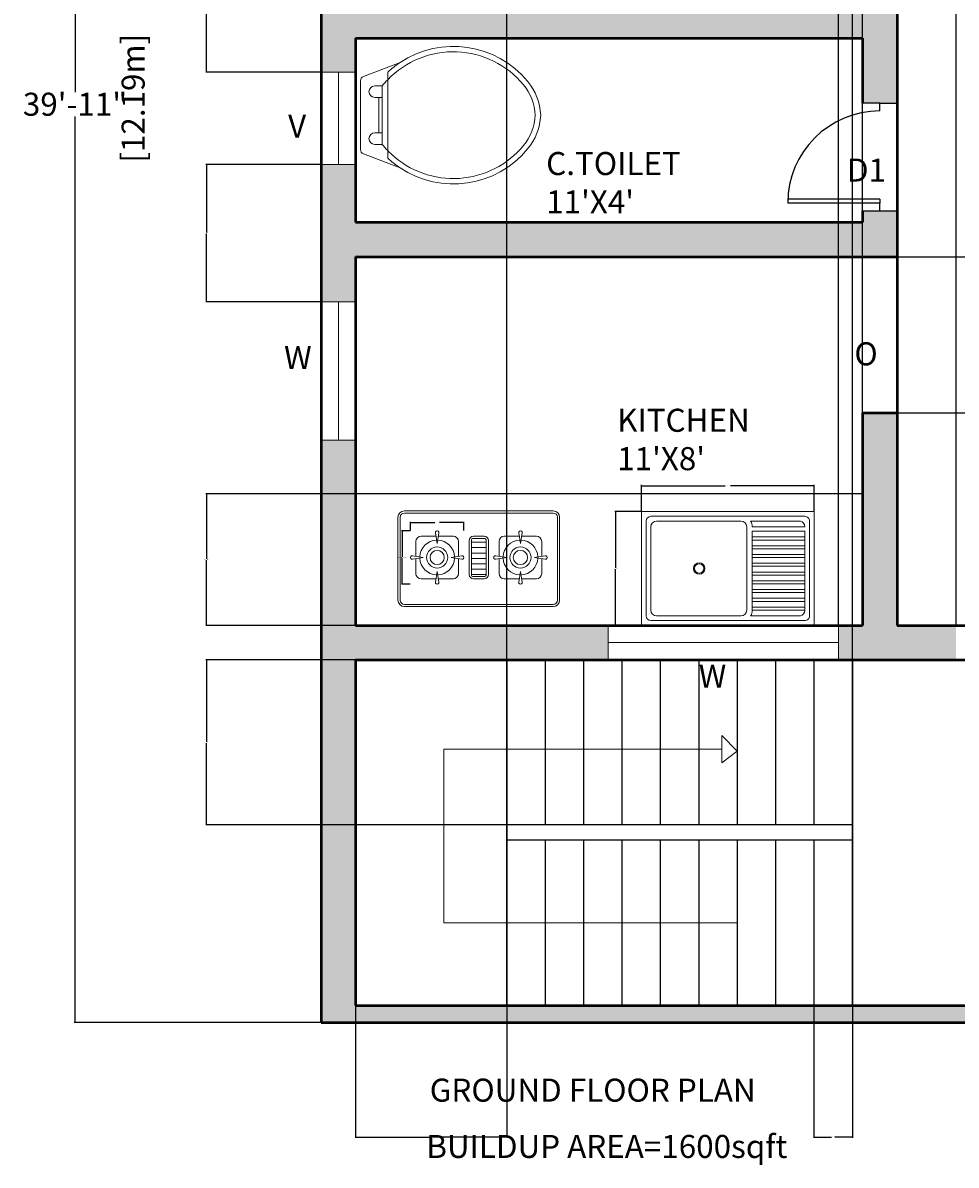
# Model space of a CAD drawing. Units: inches. Extents: x -55 to 413, y -498 to 86.
# Tile 1 of 6: x -55 to 188, y -498 to -201. Entities that reach past the tile are written whole.
import ezdxf

# ---------------------------------------------------------------- set-up
doc = ezdxf.new("R2010")
doc.units = ezdxf.units.IN
doc.header["$MEASUREMENT"] = 0
for name, color, linetype, lineweight in [('A-ANNO-DIMS', 2, 'Continuous', 18), ('A-ANNO-SYMB', 7, 'Continuous', 18), ('A-ANNO-TEXT', 7, 'Continuous', 25), ('A-AREA-IDEN', 7, 'Continuous', 25), ('A-DOOR', 3, 'Continuous', 25), ('A-EQPM', 9, 'Continuous', 18), ('A-EQPM-PATT', 9, 'Continuous', 13), ('A-FLOR-CASE', 7, 'Continuous', 25), ('A-FLOR-FIXT', 9, 'Continuous', 18), ('A-FLOR-STRS', 7, 'Continuous', 25), ('A-GLAZ', 4, 'Continuous', 18), ('A-WALL', 7, 'Continuous', 50), ('A-WALL-PATT', 8, 'Continuous', 13)]:
    doc.layers.add(name, color=color, linetype=linetype, lineweight=lineweight)
doc.styles.get("Standard").update_dxf_attribs({"font": 'arial.ttf'})
doc.dimstyles.get("Standard").update_dxf_attribs({"dimtxt": 0.18, "dimasz": 0.18, "dimexe": 0.18, "dimexo": 0.0625, "dimgap": 0.09, "dimtad": 0, "dimtih": 1, "dimtoh": 1, "dimdec": 0, "dimzin": 0, "dimdsep": 46, "dimlunit": 3, "dimtxsty": 'Standard', "dimcen": 0.09, "dimadec": 0, "dimazin": 0, "dimtfac": 1, "dimtdec": 0, "dimtofl": 0, "dimtmove": 0, "dimatfit": 3, "dimfxl": 1, "dimtolj": 1, "dimtzin": 0, "dimarcsym": 0})

# ---------------------------------------------------------------- blocks, each defined once
blk = doc.blocks.new('М12 540х820')
for p, q in [((0, 540), (-820, 540)), ((-820, 540), (-820, 0)), ((-797.5, 495), (-797.5, 45)), ((-45, 517.5), (-775, 517.5)), ((-347.5, 495), (-748, 495)), ((-301.7, 495), (-64.8, 495)), ((-22.5, 45), (-22.5, 495)), ((0, 0), (0, 540)), ((-775, 468), (-775, 72)), ((-320.5, 468), (-320.5, 72)), ((-293.7, 468), (-293.7, 472.5)), ((-293.7, 468), (-45, 468)), ((-293.7, 446.6), (-45, 446.6)), ((-293.7, 419.6), (-293.7, 446.6)), ((-45, 469.5), (-45, 468)), ((-45, 419.6), (-45, 446.6)), ((-293.7, 419.6), (-45, 419.6)), ((-293.7, 405), (-45, 405)), ((-293.7, 378), (-293.7, 405)), ((-45, 378), (-45, 405)), ((-293.7, 378), (-45, 378)), ((-293.7, 336.4), (-293.7, 363.4)), ((-293.7, 363.4), (-45, 363.4)), ((-293.7, 336.4), (-45, 336.4)), ((-45, 336.4), (-45, 363.4)), ((-293.7, 294.7), (-293.7, 321.7)), ((-293.7, 321.7), (-45, 321.7)), ((-293.7, 294.7), (-45, 294.7)), ((-293.7, 253.1), (-293.7, 280.1)), ((-293.7, 280.1), (-45, 280.1)), ((-45, 294.7), (-45, 321.7)), ((-45, 253.1), (-45, 280.1)), ((-293.7, 253.1), (-45, 253.1)), ((-293.7, 211.5), (-293.7, 238.5)), ((-293.7, 238.5), (-45, 238.5)), ((-45, 211.5), (-45, 238.5)), ((-293.7, 211.5), (-45, 211.5)), ((-293.7, 169.9), (-293.7, 196.9)), ((-293.7, 196.9), (-45, 196.9)), ((-293.7, 169.9), (-45, 169.9)), ((-45, 169.9), (-45, 196.9)), ((-293.7, 128.2), (-293.7, 155.2)), ((-293.7, 155.2), (-45, 155.2)), ((-293.7, 128.2), (-45, 128.2)), ((-293.7, 113.6), (-45, 113.6)), ((-293.7, 86.6), (-293.7, 113.6)), ((-45, 128.2), (-45, 155.2)), ((-45, 86.6), (-45, 113.6)), ((-293.7, 86.6), (-45, 86.6)), ((-293.7, 72), (-45, 72)), ((-45, 70.5), (-45, 72)), ((-820, 0), (0, 0)), ((-775, 22.5), (-45, 22.5)), ((-748, 45), (-347.5, 45)), ((-301.7, 45), (-64.8, 45))]:
    blk.add_line(p, q)
at = {"ltscale": 0.06}
for p, q in [((-820, 0), (-820, 540)), ((-820, 540), (0, 540)), ((0, 540), (0, 536.9)), ((0, 536.9), (0, 0)), ((-293.7, 446.6), (-45, 446.6)), ((-293.7, 405), (-293.7, 446.6)), ((-45, 446.6), (-45, 419.6)), ((-293.7, 363.4), (-293.7, 405)), ((-45, 419.6), (-45, 378)), ((-293.7, 321.7), (-293.7, 363.4)), ((-45, 378), (-45, 336.4)), ((-45, 336.4), (-45, 294.7)), ((-293.7, 280.1), (-293.7, 321.7)), ((-293.7, 238.5), (-293.7, 280.1)), ((-45, 294.7), (-45, 253.1)), ((-293.7, 196.9), (-293.7, 238.5)), ((-45, 253.1), (-45, 211.5)), ((-293.7, 155.2), (-293.7, 196.9)), ((-45, 211.5), (-45, 169.9)), ((-45, 169.9), (-45, 128.2)), ((-293.7, 113.6), (-293.7, 155.2)), ((-293.7, 72), (-293.7, 113.6)), ((-45, 128.2), (-45, 86.6)), ((-45, 72), (-293.7, 72)), ((-45, 86.6), (-45, 72)), ((0, 0), (-820, 0))]:
    blk.add_line(p, q, dxfattribs=at)
at = {"extrusion": (0, 0, -1)}
for centre, major_axis, start_param, end_param in [((-775, 495), (-15.9, 15.9), -0.785398, 0.785398), ((-775, 495), (-15.9, 15.9), -0.785398, 0.785398), ((-748, 468), (-19.1, -19.1), 0.785398, 2.356194), ((-748, 468), (-19.1, -19.1), 0.785398, 2.356194), ((-347.5, 468), (-19.1, 19.1), 0.785398, 2.356194), ((-347.5, 468), (-19.1, 19.1), 0.785398, 2.356194), ((-343.2, 468), (-35, 35), 1.779263, 2.356194), ((-343.2, 468), (-35, 35), 1.779263, 2.356192), ((-72.3, 468.8), (-19.3, 19.3), 1.0328, 2.38382), ((-72.3, 468.8), (-19.3, 19.3), 1.0328, 1.064673), ((-72.3, 468.8), (-19.3, 19.3), 1.064673, 2.328569), ((-45, 495), (-15.9, -15.9), 2.356194, 3.926991), ((-45, 495), (-15.9, -15.9), 2.356194, 3.926991), ((-343.2, 468), (-35, 35), 2.356192, 2.356194), ((-72.3, 468.8), (-19.3, 19.3), 2.328569, 2.38382), ((-545.5, 270), (-19.1, -19.1), 3.926991, 10.210176), ((-545.5, 270), (-19.1, -19.1), 3.926991, 10.210176), ((-545.5, 270), (-15.9, -15.9), 3.926991, 10.210176), ((-545.5, 270), (-15.9, -15.9), 3.926991, 10.210176), ((-748, 72), (-19.1, 19.1), 3.926991, 5.497787), ((-748, 72), (-19.1, 19.1), 3.926991, 5.497787), ((-347.5, 72), (-19.1, -19.1), 3.926991, 5.497787), ((-347.5, 72), (-19.1, -19.1), 3.926991, 5.497787), ((-343.2, 72), (-35, -35), 3.926991, 4.503922), ((-343.2, 72), (-35, -35), 3.926991, 4.503922), ((-72.3, 71.2), (-19.3, -19.3), 3.899365, 5.250385), ((-72.3, 71.2), (-19.3, -19.3), 3.954617, 5.218512), ((-72.3, 71.2), (-19.3, -19.3), 3.899365, 3.954617), ((-775, 45), (-15.9, -15.9), 5.497787, 7.068583), ((-775, 45), (-15.9, -15.9), 5.497787, 7.068583), ((-72.3, 71.2), (-19.3, -19.3), 5.218512, 5.250385), ((-45, 45), (-15.9, 15.9), 2.356194, 3.926991), ((-45, 45), (-15.9, 15.9), 2.356194, 3.926991)]:
    blk.add_ellipse(centre, major_axis=major_axis, ratio=1, start_param=start_param, end_param=end_param, dxfattribs=at)
blk = doc.blocks.new('*D3')
at = {"layer": 'A-ANNO-DIMS', "color": 0, "lineweight": -2, "transparency": 16777216}
for p, q in [((22.94, 17.54), (-41.24, 17.54)), ((-41.06, 17.36), (-41.06, -218.55)), ((-41.06, -460.78), (-41.06, -224.87)), ((22.94, -460.96), (-41.24, -460.96))]:
    blk.add_line(p, q, dxfattribs=at)
at = {"layer": 'A-ANNO-DIMS', "color": 0, "transparency": 16777216}
for points in [[(-41.09, 17.36), (-41.03, 17.36), (-41.06, 17.54)], [(-41.09, -460.78), (-41.03, -460.78), (-41.06, -460.96)]]:
    blk.add_solid(points, dxfattribs=at)
at = {"layer": 'Defpoints', "color": 0, "transparency": 16777216}
for p in [(23, 17.54), (-41.06, -460.96), (23, -460.96)]:
    blk.add_point(p, dxfattribs=at)
at = {"layer": 'A-ANNO-DIMS', "color": 0, "transparency": 16777216, "insert": (-41.06, -221.71), "char_height": 6, "attachment_point": 5}
blk.add_mtext('\\A1;39\'-11"', dxfattribs=at)
blk = doc.blocks.new('WC-PLAN')
for p, q in [((7.1, 27.15), (7.1, 29.12)), ((7.1, 27.15), (7.1, 17.92)), ((7.1, 8.69), (7.1, 17.92)), ((7.1, 6.73), (7.1, 8.69))]:
    blk.add_line(p, q)
for points in [[(10.32, 31.66, -0.383919), (43.53, 26.74, -0.163732), (46.92, 17.92, -0.359733)], [(7.1, 27.15, -0.448546), (42.45, 25.85, -0.162618), (45.51, 17.92, -0.470877)], [(0, 17.92), (0, 26.88, -0.31031), (0.75, 27.98), (10.32, 31.66, -0.209071)], [(7.1, 29.12, -0.040937), (10.32, 31.66, -0.163732)], [(5.69, 25.54, -0.022712), (7.1, 27.15, -0.162618)], [(5.69, 25.54), (3.72, 25.54, 1), (3.72, 22.54), (4.74, 22.54)], [(5.69, 17.92), (5.69, 25.54, -0.476108)], [(0, 17.92), (0, 8.97, 0.31031), (0.75, 7.87), (10.32, 4.19, 0.209071)], [(5.69, 17.92), (5.69, 10.31, 0.022712)], [(8.06, 7.75, 0.431639), (42.45, 10, 0.162618), (45.51, 17.92, 0.470877)], [(10.32, 4.19, 0.383919), (43.53, 9.11, 0.163732), (46.92, 17.92, 0.359733)], [(5.69, 10.31), (3.72, 10.31, -1), (3.72, 13.31), (4.74, 13.31)], [(5.69, 10.31, 0.022712), (7.1, 8.69, 0.162618)], [(7.1, 8.69, 0.014165), (8.06, 7.75, 0.162618)], [(7.1, 6.73, 0.040937), (10.32, 4.19, 0.163732)]]:
    blk.add_lwpolyline(points, format="xyb")
for points in [[(4.74, 22.54), (4.74, 13.31)], [(4.74, 22.54), (5.69, 22.54)], [(4.74, 13.31), (5.69, 13.31)]]:
    blk.add_lwpolyline(points)
blk = doc.blocks.new('DOOR-SINGLE-24')
for p, q in [((24, 28), (19.5, 28)), ((24, 26), (24, 28)), ((24, 28), (28.5, 28)), ((24, 3), (0, 3)), ((24, 3), (24, 2)), ((24, 2), (0, 2)), ((24, 0), (24, 2)), ((19.5, 0), (28.5, 0))]:
    blk.add_line(p, q)
blk.add_arc((24, 2), 24, 90, 180)
blk = doc.blocks.new('COOKTOP-BURNER')
for p, q in [((6.66, 12.49), (2.75, 12.49)), ((6.52, 13.4), (6.96, 10.59)), ((6.96, 10.59), (7.4, 13.4)), ((11.17, 12.49), (7.26, 12.49)), ((1.42, 11.17), (1.42, 7.26)), ((12.5, 7.26), (12.5, 11.17)), ((0.52, 7.4), (3.33, 6.96)), ((3.33, 6.96), (0.52, 6.52)), ((1.42, 6.66), (1.42, 2.75)), ((13.4, 7.4), (10.59, 6.96)), ((10.59, 6.96), (13.4, 6.52)), ((12.5, 2.75), (12.5, 6.66)), ((6.52, 0.52), (6.96, 3.33)), ((6.96, 3.33), (7.4, 0.52)), ((2.75, 1.42), (6.66, 1.42)), ((7.26, 1.42), (11.17, 1.42))]:
    blk.add_line(p, q)
for radius in [2.75, 1.86]:
    blk.add_circle((6.96, 6.96), radius)
for centre, radius, start, end in [((2.75, 11.17), 1.33, 90, 180), ((6.96, 13.47), 0.448, 351.0363, 188.9637), ((11.17, 11.17), 1.33, 0, 90), ((6.96, 6.96), 4.52, 91.7678, 178.2322), ((6.96, 6.96), 4.52, 1.7678, 88.2322), ((0.45, 6.96), 0.448, 81.0363, 278.9637), ((6.96, 6.96), 4.52, 181.7678, 268.2322), ((6.96, 6.96), 4.52, 271.7678, 358.2322), ((13.47, 6.96), 0.448, 261.0363, 98.9637), ((2.75, 2.75), 1.33, 180, 270), ((6.96, 0.45), 0.448, 171.0363, 8.9637), ((11.17, 2.75), 1.33, 270, 0)]:
    blk.add_arc(centre, radius, start, end)
blk = doc.blocks.new('WIN-60IN')
for p, q in [((0, 9), (60, 9)), ((0, 0), (0, 9)), ((60, 9), (60, 0)), ((0, 4.5), (60, 4.5)), ((60, 0), (0, 0))]:
    blk.add_line(p, q)
blk = doc.blocks.new('WIN-24IN')
for p, q in [((24, 9), (0, 9)), ((0, 9), (0, 0)), ((24, 0), (24, 9)), ((0, 4.5), (24, 4.5)), ((0, 0), (24, 0))]:
    blk.add_line(p, q)
blk = doc.blocks.new('WIN-36IN')
for p, q in [((0, 36), (0, 0)), ((9, 36), (0, 36)), ((4.5, 36), (4.5, 0)), ((9, 0), (9, 36)), ((0, 0), (9, 0))]:
    blk.add_line(p, q)
blk = doc.blocks.new('*D23')
at = {"layer": 'A-ANNO-DIMS', "color": 0, "lineweight": -2, "transparency": 16777216}
for p, q in [((46.18, -332.81), (43.97, -332.81)), ((44.15, -332.99), (44.15, -339.61)), ((44.15, -346.59), (44.15, -339.97)), ((46.18, -346.77), (43.97, -346.77))]:
    blk.add_line(p, q, dxfattribs=at)
at = {"layer": 'A-ANNO-DIMS', "color": 0, "transparency": 16777216}
for points in [[(44.12, -332.99), (44.18, -332.99), (44.15, -332.81)], [(44.12, -346.59), (44.18, -346.59), (44.15, -346.77)]]:
    blk.add_solid(points, dxfattribs=at)
at = {"layer": 'Defpoints', "color": 0, "transparency": 16777216}
for p in [(44.15, -332.81), (46.25, -332.81), (46.25, -346.77)]:
    blk.add_point(p, dxfattribs=at)
at = {"layer": 'A-ANNO-DIMS', "color": 0, "transparency": 16777216, "insert": (44.15, -339.79), "char_height": 0.18, "attachment_point": 5}
blk.add_mtext('\\A1;BURNER 1\'-2" TYP.', dxfattribs=at)
blk = doc.blocks.new('*D24')
at = {"layer": 'A-ANNO-DIMS', "color": 0, "lineweight": -2, "transparency": 16777216}
for p, q in [((46.25, -332.75), (46.25, -330.53)), ((46.43, -330.71), (52.6, -330.71)), ((60.03, -330.71), (53.86, -330.71)), ((60.21, -332.75), (60.21, -330.53))]:
    blk.add_line(p, q, dxfattribs=at)
at = {"layer": 'A-ANNO-DIMS', "color": 0, "transparency": 16777216}
for points in [[(46.43, -330.68), (46.43, -330.74), (46.25, -330.71)], [(60.03, -330.68), (60.03, -330.74), (60.21, -330.71)]]:
    blk.add_solid(points, dxfattribs=at)
at = {"layer": 'Defpoints', "color": 0, "transparency": 16777216}
for p in [(46.25, -332.81), (60.21, -330.71), (60.21, -332.81)]:
    blk.add_point(p, dxfattribs=at)
at = {"layer": 'A-ANNO-DIMS', "color": 0, "transparency": 16777216, "insert": (53.23, -330.71), "char_height": 0.18, "attachment_point": 5}
blk.add_mtext('\\A1;1\'-2" TYP.', dxfattribs=at)
blk = doc.blocks.new('*D25')
at = {"layer": 'A-ANNO-DIMS', "color": 0, "lineweight": -2, "transparency": 16777216}
for p, q in [((106.4, -327.76), (106.4, -320.9)), ((106.58, -321.08), (128.24, -321.08)), ((151.22, -321.08), (129.56, -321.08)), ((151.4, -327.76), (151.4, -320.9))]:
    blk.add_line(p, q, dxfattribs=at)
at = {"layer": 'A-ANNO-DIMS', "color": 0, "transparency": 16777216}
for points in [[(106.58, -321.05), (106.58, -321.11), (106.4, -321.08)], [(151.22, -321.05), (151.22, -321.11), (151.4, -321.08)]]:
    blk.add_solid(points, dxfattribs=at)
at = {"layer": 'Defpoints', "color": 0, "transparency": 16777216}
for p in [(151.4, -321.08), (106.4, -327.83), (151.4, -327.83)]:
    blk.add_point(p, dxfattribs=at)
at = {"layer": 'A-ANNO-DIMS', "color": 0, "transparency": 16777216, "insert": (128.9, -321.08), "char_height": 0.18, "attachment_point": 5}
blk.add_mtext('\\A1;SINK 3\'-9"', dxfattribs=at)
blk = doc.blocks.new('*D26')
at = {"layer": 'A-ANNO-DIMS', "color": 0, "lineweight": -2, "transparency": 16777216}
for p, q in [((106.34, -327.83), (99.47, -327.83)), ((99.65, -328.01), (99.65, -342.46)), ((99.65, -357.28), (99.65, -342.83)), ((106.34, -357.46), (99.47, -357.46))]:
    blk.add_line(p, q, dxfattribs=at)
at = {"layer": 'A-ANNO-DIMS', "color": 0, "transparency": 16777216}
for points in [[(99.62, -328.01), (99.68, -328.01), (99.65, -327.83)], [(99.62, -357.28), (99.68, -357.28), (99.65, -357.46)]]:
    blk.add_solid(points, dxfattribs=at)
at = {"layer": 'Defpoints', "color": 0, "transparency": 16777216}
for p in [(99.65, -327.83), (106.4, -327.83), (106.4, -357.46)]:
    blk.add_point(p, dxfattribs=at)
at = {"layer": 'A-ANNO-DIMS', "color": 0, "transparency": 16777216, "insert": (99.65, -342.64), "char_height": 0.18, "attachment_point": 5}
blk.add_mtext('\\A1;2\'-5 1/2"', dxfattribs=at)
blk = doc.blocks.new('*D31')
at = {"layer": 'A-ANNO-DIMS', "color": 0, "lineweight": -2, "transparency": 16777216}
for p, q in [((22.94, -237.4), (-6.98, -237.4)), ((-6.8, -237.58), (-6.8, -255.13)), ((-6.8, -273.04), (-6.8, -255.5)), ((22.94, -273.22), (-6.98, -273.22))]:
    blk.add_line(p, q, dxfattribs=at)
at = {"layer": 'A-ANNO-DIMS', "color": 0, "transparency": 16777216}
for points in [[(-6.83, -237.58), (-6.77, -237.58), (-6.8, -237.4)], [(-6.83, -273.04), (-6.77, -273.04), (-6.8, -273.22)]]:
    blk.add_solid(points, dxfattribs=at)
at = {"layer": 'Defpoints', "color": 0, "transparency": 16777216}
for p in [(23, -237.4), (-6.8, -273.22), (23, -273.22)]:
    blk.add_point(p, dxfattribs=at)
at = {"layer": 'A-ANNO-DIMS', "color": 0, "transparency": 16777216, "insert": (-6.8, -255.31), "char_height": 0.18, "attachment_point": 5}
blk.add_mtext('\\A1;3\'-0"', dxfattribs=at)
blk = doc.blocks.new('*D32')
at = {"layer": 'A-ANNO-DIMS', "color": 0, "lineweight": -2, "transparency": 16777216}
for p, q in [((22.94, -154.08), (-6.98, -154.08)), ((-6.8, -154.26), (-6.8, -183.56)), ((-6.8, -213.22), (-6.8, -183.93)), ((22.94, -213.4), (-6.98, -213.4))]:
    blk.add_line(p, q, dxfattribs=at)
at = {"layer": 'A-ANNO-DIMS', "color": 0, "transparency": 16777216}
for points in [[(-6.83, -154.26), (-6.77, -154.26), (-6.8, -154.08)], [(-6.83, -213.22), (-6.77, -213.22), (-6.8, -213.4)]]:
    blk.add_solid(points, dxfattribs=at)
at = {"layer": 'Defpoints', "color": 0, "transparency": 16777216}
for p in [(23, -154.08), (-6.8, -213.4), (23, -213.4)]:
    blk.add_point(p, dxfattribs=at)
at = {"layer": 'A-ANNO-DIMS', "color": 0, "transparency": 16777216, "insert": (-6.8, -183.74), "char_height": 0.18, "attachment_point": 5}
blk.add_mtext('\\A1;4\'-11 1/2"', dxfattribs=at)
blk = doc.blocks.new('*D35')
at = {"layer": 'A-ANNO-DIMS', "color": 0, "lineweight": -2, "transparency": 16777216}
for p, q in [((164.07, -261.46), (412.98, -261.46)), ((412.8, -261.64), (412.8, -281.58)), ((412.8, -301.89), (412.8, -281.95)), ((164.07, -302.07), (412.98, -302.07))]:
    blk.add_line(p, q, dxfattribs=at)
at = {"layer": 'A-ANNO-DIMS', "color": 0, "transparency": 16777216}
for points in [[(412.77, -261.64), (412.83, -261.64), (412.8, -261.46)], [(412.77, -301.89), (412.83, -301.89), (412.8, -302.07)]]:
    blk.add_solid(points, dxfattribs=at)
at = {"layer": 'Defpoints', "color": 0, "transparency": 16777216}
for p in [(164, -261.46), (412.8, -261.46), (164, -302.07)]:
    blk.add_point(p, dxfattribs=at)
at = {"layer": 'A-ANNO-DIMS', "color": 0, "transparency": 16777216, "insert": (412.8, -281.76), "char_height": 0.18, "attachment_point": 5}
blk.add_mtext('\\A1;3\'-4 1/2"', dxfattribs=at)
blk = doc.blocks.new('*D40')
at = {"layer": 'A-ANNO-DIMS', "color": 0, "lineweight": -2, "transparency": 16777216}
for p, q in [((157.71, -357.4), (157.71, 47.52)), ((157.89, 47.34), (160.32, 47.34)), ((163.82, 47.34), (161.39, 47.34)), ((164, -357.4), (164, 47.52))]:
    blk.add_line(p, q, dxfattribs=at)
at = {"layer": 'A-ANNO-DIMS', "color": 0, "transparency": 16777216}
for points in [[(157.89, 47.37), (157.89, 47.31), (157.71, 47.34)], [(163.82, 47.37), (163.82, 47.31), (164, 47.34)]]:
    blk.add_solid(points, dxfattribs=at)
at = {"layer": 'Defpoints', "color": 0, "transparency": 16777216}
for p in [(164, 47.34), (157.71, -357.46), (164, -357.46)]:
    blk.add_point(p, dxfattribs=at)
at = {"layer": 'A-ANNO-DIMS', "color": 0, "transparency": 16777216, "insert": (160.86, 47.34), "char_height": 0.18, "attachment_point": 5}
blk.add_mtext('\\A1;0\'-6 1/2"', dxfattribs=at)
blk = doc.blocks.new('*D41')
at = {"layer": 'A-ANNO-DIMS', "color": 0, "lineweight": -2, "transparency": 16777216}
for p, q in [((173, -357.4), (173, 47.52)), ((173.18, 47.34), (180.15, 47.34)), ((188.17, 47.34), (181.21, 47.34)), ((188.35, -357.4), (188.35, 47.52))]:
    blk.add_line(p, q, dxfattribs=at)
at = {"layer": 'A-ANNO-DIMS', "color": 0, "transparency": 16777216}
for points in [[(173.18, 47.37), (173.18, 47.31), (173, 47.34)], [(188.17, 47.37), (188.17, 47.31), (188.35, 47.34)]]:
    blk.add_solid(points, dxfattribs=at)
at = {"layer": 'Defpoints', "color": 0, "transparency": 16777216}
for p in [(188.35, 47.34), (173, -357.46), (188.35, -357.46)]:
    blk.add_point(p, dxfattribs=at)
at = {"layer": 'A-ANNO-DIMS', "color": 0, "transparency": 16777216, "insert": (180.68, 47.34), "char_height": 0.18, "attachment_point": 5}
blk.add_mtext('\\A1;1\'-3 1/2"', dxfattribs=at)
blk = doc.blocks.new('*D43')
at = {"layer": 'A-ANNO-DIMS', "color": 0, "lineweight": -2, "transparency": 16777216}
for p, q in [((71.33, -456.4), (71.33, 47.52)), ((71.51, 47.34), (116, 47.34)), ((161.15, 47.34), (116.66, 47.34)), ((161.33, -456.4), (161.33, 47.52))]:
    blk.add_line(p, q, dxfattribs=at)
at = {"layer": 'A-ANNO-DIMS', "color": 0, "transparency": 16777216}
for points in [[(71.51, 47.37), (71.51, 47.31), (71.33, 47.34)], [(161.15, 47.37), (161.15, 47.31), (161.33, 47.34)]]:
    blk.add_solid(points, dxfattribs=at)
at = {"layer": 'Defpoints', "color": 0, "transparency": 16777216}
for p in [(161.33, 47.34), (71.33, -456.46), (161.33, -456.46)]:
    blk.add_point(p, dxfattribs=at)
at = {"layer": 'A-ANNO-DIMS', "color": 0, "transparency": 16777216, "insert": (116.33, 47.34), "char_height": 0.18, "attachment_point": 5}
blk.add_mtext('\\A1;7\'-6"', dxfattribs=at)
blk = doc.blocks.new('*D44')
at = {"layer": 'A-ANNO-DIMS', "color": 0, "lineweight": -2, "transparency": 16777216}
for p, q in [((32, -456.52), (32, -490.94)), ((71.33, -456.52), (71.33, -490.94)), ((32.18, -490.76), (51.13, -490.76)), ((71.15, -490.76), (52.21, -490.76))]:
    blk.add_line(p, q, dxfattribs=at)
at = {"layer": 'A-ANNO-DIMS', "color": 0, "transparency": 16777216}
for points in [[(32.18, -490.73), (32.18, -490.79), (32, -490.76)], [(71.15, -490.73), (71.15, -490.79), (71.33, -490.76)]]:
    blk.add_solid(points, dxfattribs=at)
at = {"layer": 'Defpoints', "color": 0, "transparency": 16777216}
for p in [(32, -456.46), (71.33, -456.46), (71.33, -490.76)]:
    blk.add_point(p, dxfattribs=at)
at = {"layer": 'A-ANNO-DIMS', "color": 0, "transparency": 16777216, "insert": (51.67, -490.76), "char_height": 0.18, "attachment_point": 5}
blk.add_mtext('\\A1;3\'-3 1/2"', dxfattribs=at)
blk = doc.blocks.new('*D45')
at = {"layer": 'A-ANNO-DIMS', "color": 0, "lineweight": -2, "transparency": 16777216}
for p, q in [((151.33, -456.52), (151.33, -490.94)), ((161.33, -456.52), (161.33, -490.94)), ((151.51, -490.76), (155.93, -490.76)), ((161.15, -490.76), (156.73, -490.76))]:
    blk.add_line(p, q, dxfattribs=at)
at = {"layer": 'A-ANNO-DIMS', "color": 0, "transparency": 16777216}
for points in [[(151.51, -490.73), (151.51, -490.79), (151.33, -490.76)], [(161.15, -490.73), (161.15, -490.79), (161.33, -490.76)]]:
    blk.add_solid(points, dxfattribs=at)
at = {"layer": 'Defpoints', "color": 0, "transparency": 16777216}
for p in [(151.33, -456.46), (161.33, -456.46), (161.33, -490.76)]:
    blk.add_point(p, dxfattribs=at)
at = {"layer": 'A-ANNO-DIMS', "color": 0, "transparency": 16777216, "insert": (156.33, -490.76), "char_height": 0.18, "attachment_point": 5}
blk.add_mtext('\\A1;0\'-10"', dxfattribs=at)
blk = doc.blocks.new('*D48')
at = {"layer": 'A-ANNO-DIMS', "color": 0, "lineweight": -2, "transparency": 16777216}
for p, q in [((71.27, -366.46), (-6.98, -366.46)), ((-6.8, -366.64), (-6.8, -387.78)), ((-6.8, -409.28), (-6.8, -388.14)), ((71.27, -409.46), (-6.98, -409.46))]:
    blk.add_line(p, q, dxfattribs=at)
at = {"layer": 'A-ANNO-DIMS', "color": 0, "transparency": 16777216}
for points in [[(-6.83, -366.64), (-6.77, -366.64), (-6.8, -366.46)], [(-6.83, -409.28), (-6.77, -409.28), (-6.8, -409.46)]]:
    blk.add_solid(points, dxfattribs=at)
at = {"layer": 'Defpoints', "color": 0, "transparency": 16777216}
for p in [(-6.8, -366.46), (71.33, -366.46), (71.33, -409.46)]:
    blk.add_point(p, dxfattribs=at)
at = {"layer": 'A-ANNO-DIMS', "color": 0, "transparency": 16777216, "insert": (-6.8, -387.96), "char_height": 0.18, "attachment_point": 5}
blk.add_mtext('\\A1;3\'-7"', dxfattribs=at)
blk = doc.blocks.new('*D49')
at = {"layer": 'A-ANNO-DIMS', "color": 0, "lineweight": -2, "transparency": 16777216}
for p, q in [((31.94, -323.17), (-6.98, -323.17)), ((-6.8, -323.35), (-6.8, -340.13)), ((-6.8, -357.28), (-6.8, -340.5)), ((31.94, -357.46), (-6.98, -357.46))]:
    blk.add_line(p, q, dxfattribs=at)
at = {"layer": 'A-ANNO-DIMS', "color": 0, "transparency": 16777216}
for points in [[(-6.83, -323.35), (-6.77, -323.35), (-6.8, -323.17)], [(-6.83, -357.28), (-6.77, -357.28), (-6.8, -357.46)]]:
    blk.add_solid(points, dxfattribs=at)
at = {"layer": 'Defpoints', "color": 0, "transparency": 16777216}
for p in [(32, -323.17), (-6.8, -357.46), (32, -357.46)]:
    blk.add_point(p, dxfattribs=at)
at = {"layer": 'A-ANNO-DIMS', "color": 0, "transparency": 16777216, "insert": (-6.8, -340.31), "char_height": 0.18, "attachment_point": 5}
blk.add_mtext('\\A1;2\'-10 1/2"', dxfattribs=at)

msp = doc.modelspace()

# ---------------------------------------------------------------- hatches: boundary and pattern name
at = {"layer": 'A-EQPM-PATT'}
h = msp.add_hatch(dxfattribs=at)
h.set_pattern_fill('ANSI31', color=256, scale=11.2404, angle=-45, style=0)
h.paths.add_polyline_path([(66.02, -335.36), (66.01, -335.29), (66, -335.22), (65.97, -335.15), (65.94, -335.09), (65.9, -335.03), (65.85, -334.97), (65.8, -334.92), (65.74, -334.88), (65.67, -334.85), (65.61, -334.83), (65.54, -334.81), (65.46, -334.81), (62.68, -334.81), (62.61, -334.81), (62.54, -334.83), (62.47, -334.85), (62.4, -334.88), (62.34, -334.92), (62.29, -334.97), (62.24, -335.03), (62.2, -335.09), (62.17, -335.15), (62.15, -335.22), (62.13, -335.29), (62.13, -335.36), (62.13, -344.22), (62.13, -344.29), (62.15, -344.36), (62.17, -344.43), (62.2, -344.5), (62.24, -344.56), (62.29, -344.61), (62.34, -344.66), (62.4, -344.7), (62.47, -344.73), (62.54, -344.76), (62.61, -344.77), (62.68, -344.77), (65.46, -344.77), (65.54, -344.77), (65.61, -344.76), (65.67, -344.73), (65.74, -344.7), (65.8, -344.66), (65.85, -344.61), (65.9, -344.56), (65.94, -344.5), (65.97, -344.43), (66, -344.36), (66.01, -344.29), (66.02, -344.22)])
at = {"layer": 'A-WALL-PATT'}
h = msp.add_hatch(color=256, dxfattribs=at)
h.dxf.hatch_style = 1
h.paths.add_polyline_path([(97.55, 17.54), (23, 17.54), (23, -94.08), (32, -94.08), (32, 8.54), (97.55, 8.54)])
h.paths.add_polyline_path([(191, 17.54), (157.55, 17.54), (157.55, 8.54), (164, 8.54), (164, -80.46), (168.5, -80.46), (173, -80.46), (173, 8.54), (191, 8.54)])
h.paths.add_polyline_path([(312.03, 17.54), (215, 17.54), (215, 8.54), (233, 8.54), (233, -111.46), (173, -111.46), (173, -108.46), (164, -108.46), (164, -164.46), (168.5, -164.46), (173, -164.46), (173, -120.46), (233, -120.46), (233, -164.46), (237.5, -164.46), (242, -164.46), (242, 8.54), (312.03, 8.54)])
h.paths.add_polyline_path([(383, 17.54), (372.03, 17.54), (372.03, 8.54), (374, 8.54), (374, -99.01), (383, -99.01)])
h.paths.add_polyline_path([(383, -159.01), (374, -159.01), (374, -195.46), (242, -195.46), (242, -192.46), (233, -192.46), (233, -204.46), (374, -204.46), (374, -224.71), (383, -224.71)])
h.paths.add_polyline_path([(173, -192.46), (164, -192.46), (164, -195.46), (32, -195.46), (32, -154.08), (23, -154.08), (23, -213.4), (32, -213.4), (32, -204.46), (164, -204.46), (164, -221.46), (168.5, -221.46), (173, -221.46)])
h.paths.add_polyline_path([(173, -249.46), (164, -249.46), (164, -252.46), (32, -252.46), (32, -237.4), (23, -237.4), (23, -273.22), (32, -273.22), (32, -261.46), (164, -261.46), (173, -261.46)])
h.paths.add_polyline_path([(32, -309.22), (23, -309.22), (23, -456.46), (23, -460.96), (199.52, -460.96), (199.52, -456.46), (32, -456.46), (32, -366.46), (97.71, -366.46), (97.71, -357.46), (32, -357.46)])
h.paths.add_polyline_path([(188.35, -357.46), (173, -357.46), (173, -302.07), (164, -302.07), (164, -357.46), (157.71, -357.46), (157.71, -366.46), (188.35, -366.46)])
h.paths.add_polyline_path([(223.25, -357.46), (212.35, -357.46), (212.35, -366.46), (223.25, -366.46), (223.25, -361.96)])
h.paths.add_polyline_path([(287.63, -357.46), (271.25, -357.46), (271.25, -361.96), (271.25, -366.46), (287.63, -366.46)])
h.paths.add_polyline_path([(374, -357.46), (311.63, -357.46), (311.63, -366.46), (374, -366.46)])
h.paths.add_polyline_path([(383, -456.46), (383, -366.46), (378.5, -366.46), (378.5, -456.46), (309.45, -456.46), (309.45, -460.96), (383, -460.96)])
h.paths.add_polyline_path([(309.45, -458.71), (199.52, -458.71), (199.52, -460.96), (309.45, -460.96)])
h.paths.add_polyline_path([(383, -260.71), (374, -260.71), (374, -280.96), (371, -280.96), (371, -285.46), (374, -285.46), (374, -366.46), (383, -366.46)])
h.paths.add_polyline_path([(343, -283.21), (343, -280.96), (321.5, -280.96), (321.5, -357.46), (326, -357.46), (326, -285.46), (343, -285.46)])

# ---------------------------------------------------------------- linework, layer by layer
at = {"layer": 'A-ANNO-SYMB'}
for p, q in [((127.33, -389.71), (127.33, -386.13)), ((127.33, -386.13), (131.33, -390.23)), ((54.95, -434.96), (54.95, -389.71)), ((54.95, -389.71), (127.33, -389.71)), ((127.33, -389.71), (127.33, -393.29)), ((127.33, -393.29), (131.33, -390.23)), ((131.33, -434.96), (54.95, -434.96))]:
    msp.add_line(p, q, dxfattribs=at)
at = {"layer": 'A-EQPM'}
for p, q in [((43.03, -329.31), (43.03, -350.9)), ((43.59, -329.31), (43.59, -350.9)), ((83.45, -327.65), (44.69, -327.65)), ((83.45, -328.2), (44.69, -328.2)), ((84.56, -350.9), (84.56, -329.31)), ((85.11, -350.9), (85.11, -329.31)), ((61.57, -344.22), (61.57, -335.36)), ((62.13, -344.22), (62.13, -335.36)), ((62.68, -334.26), (65.46, -334.26)), ((62.68, -334.81), (65.46, -334.81)), ((66.02, -335.36), (66.02, -344.22)), ((66.57, -335.36), (66.57, -344.22)), ((65.46, -344.77), (62.68, -344.77)), ((65.46, -345.33), (62.68, -345.33)), ((44.69, -352.01), (83.45, -352.01)), ((44.69, -352.56), (83.45, -352.56))]:
    msp.add_line(p, q, dxfattribs=at)
for centre, radius, start, end in [((44.69, -329.31), 1.66, 90, 180), ((44.69, -329.31), 1.11, 90, 180), ((83.45, -329.31), 1.66, 0, 90), ((83.45, -329.31), 1.11, 0, 90), ((62.68, -335.36), 1.11, 90, 180), ((62.68, -335.36), 0.554, 90, 180), ((65.46, -335.36), 1.11, 0, 90), ((65.46, -335.36), 0.554, 0, 90), ((62.68, -344.22), 1.11, 180, 270), ((62.68, -344.22), 0.554, 180, 270), ((65.46, -344.22), 0.554, 270, 0), ((65.46, -344.22), 1.11, 270, 0), ((44.69, -350.9), 1.66, 180, 270), ((44.69, -350.9), 1.11, 180, 270), ((83.45, -350.9), 1.11, 270, 0), ((83.45, -350.9), 1.66, 270, 0)]:
    msp.add_arc(centre, radius, start, end, dxfattribs=at)
at = {"layer": 'A-FLOR-CASE'}
msp.add_line((164, -323.17), (32, -323.17), dxfattribs=at)
at = {"layer": 'A-FLOR-STRS'}
for p, q in [((71.33, -366.46), (71.33, -456.46)), ((81.33, -366.46), (81.33, -409.46)), ((91.33, -366.46), (91.33, -409.46)), ((101.33, -366.46), (101.33, -409.46)), ((111.33, -366.46), (111.33, -409.46)), ((121.33, -366.46), (121.33, -409.46)), ((131.33, -366.46), (131.33, -409.46)), ((141.33, -366.46), (141.33, -409.46)), ((151.33, -366.46), (151.33, -409.46)), ((161.33, -366.46), (161.33, -456.46)), ((161.33, -409.46), (71.33, -409.46)), ((161.33, -413.46), (71.33, -413.46)), ((81.33, -413.46), (81.33, -456.46)), ((91.33, -413.46), (91.33, -456.46)), ((101.33, -413.46), (101.33, -456.46)), ((111.33, -413.46), (111.33, -456.46)), ((121.33, -413.46), (121.33, -456.46)), ((131.33, -413.46), (131.33, -456.46)), ((141.33, -413.46), (141.33, -456.46)), ((151.33, -413.46), (151.33, -456.46))]:
    msp.add_line(p, q, dxfattribs=at)
at = {"layer": 'A-WALL'}
for p, q in [((23, 17.54), (23, -456.46)), ((173, -120.46), (173, -357.46)), ((32, -204.46), (164, -204.46)), ((32, -204.46), (32, -252.46)), ((164, -204.46), (164, -221.46)), ((164, -249.46), (164, -252.46)), ((32, -252.46), (164, -252.46)), ((32, -261.46), (164, -261.46)), ((32, -261.46), (32, -357.46)), ((164, -261.46), (173, -261.46)), ((164, -302.07), (164, -357.46)), ((164, -302.07), (173, -302.07)), ((32, -357.46), (164, -357.46)), ((173, -357.46), (223.25, -357.46)), ((173, -357.46), (223.25, -357.46)), ((32, -366.46), (223.25, -366.46)), ((32, -366.46), (32, -456.46)), ((23, -456.46), (23, -460.96)), ((32, -456.46), (199.52, -456.46)), ((23, -460.96), (383, -460.96))]:
    msp.add_line(p, q, dxfattribs=at)

# ---------------------------------------------------------------- block references
at = {"layer": 'A-DOOR'}
msp.add_blockref('DOOR-SINGLE-24', (144.5, -249.46), dxfattribs=at)
at = {"layer": 'A-EQPM'}
for p in [(46.27, -346.75), (67.95, -346.75)]:
    msp.add_blockref('COOKTOP-BURNER', p, dxfattribs=at)
at = {"layer": 'A-FLOR-FIXT'}
msp.add_blockref('WC-PLAN', (33.26, -242.48), dxfattribs=at)
at = {"layer": 'A-FLOR-FIXT', "xscale": 0.0548780487804878, "yscale": 0.0548780487804878, "zscale": 0.0548780487804878}
msp.add_blockref('М12 540х820', (151.4, -357.46), dxfattribs=at)
at = {"layer": 'A-GLAZ', "rotation": 269.9999999999999}
msp.add_blockref('WIN-24IN', (23, -213.4), dxfattribs=at)
at = {"layer": 'A-GLAZ'}
for name, p in [('WIN-36IN', (23, -309.22)), ('WIN-60IN', (97.71, -366.46))]:
    msp.add_blockref(name, p, dxfattribs=at)

# ---------------------------------------------------------------- texts
at = {"layer": 'A-ANNO-DIMS', "insert": (-28.93, -236.94), "char_height": 6, "attachment_point": 1, "rotation": 90}
msp.add_mtext('[12.19m]', dxfattribs=at)
at = {"layer": 'A-ANNO-TEXT', "char_height": 6, "attachment_point": 1}
for s, insert in [('V', (14.41, -224.39)), ('D1', (159.92, -235.86)), ('W', (13.37, -284.72)), ('O', (161.86, -283.73)), ('W', (121.32, -367.68)), ('GROUND FLOOR PLAN', (51.3, -475.55)), ('BUILDUP AREA=1600sqft', (50.4, -490.21))]:
    msp.add_mtext(s, dxfattribs=dict(at, insert=insert))
at = {"layer": 'A-AREA-IDEN', "char_height": 6, "attachment_point": 1}
for s, insert in [("C.TOILET\\P11'X4'", (81.61, -234.16)), ("KITCHEN\\P11'X8'", (100.1, -301.04))]:
    msp.add_mtext(s, dxfattribs=dict(at, insert=insert))

# ---------------------------------------------------------------- dimensions: what is measured, and where the dimension line sits
at = {"layer": 'A-ANNO-DIMS'}
for base, p1, p2, picture, middle in [((161.33, 47.34), (71.33, -456.46), (161.33, -456.46), '*D43', (116.33, 47.34)), ((164, 47.34), (157.71, -357.46), (164, -357.46), '*D40', (160.86, 47.34)), ((188.3509, 47.3397), (173.0027, -357.4603), (188.3509, -357.4603), '*D41', (180.6768, 47.3397)), ((71.33, -490.76), (32, -456.46), (71.33, -456.46), '*D44', (51.67, -490.76)), ((161.33, -490.76), (151.33, -456.46), (161.33, -456.46), '*D45', (156.33, -490.76))]:
    dim = msp.add_linear_dim(base=base, p1=p1, p2=p2, dimstyle='Standard', override={"dimdec": 1, "dimlfac": 1, "dimrnd": 0, "dimzin": 1, "dimdsep": 46, "dimlunit": 4, "dimfrac": 2}, dxfattribs=at)
    dim.commit()
    dim.dimension.update_dxf_attribs({"geometry": picture, "text_midpoint": middle})
for base, p1, p2, override, picture, middle in [((-41.05729825, -460.96025605), (23.00267102, 17.53974395), (23.00267102, -460.96025605), {"dimtxt": 6, "dimclrd": 0, "dimclre": 0, "dimclrt": 0}, '*D3', (-41.05729825, -221.71025605)), ((-6.8, -213.4), (23, -154.08), (23, -213.4), {"dimdec": 1, "dimlfac": 1, "dimrnd": 0, "dimzin": 1, "dimdsep": 46, "dimlunit": 4, "dimfrac": 2}, '*D32', (-6.8, -183.74)), ((-6.8, -273.22), (23, -237.4), (23, -273.22), {"dimdec": 1, "dimlfac": 1, "dimrnd": 0, "dimzin": 1, "dimdsep": 46, "dimlunit": 4, "dimfrac": 2}, '*D31', (-6.8, -255.31)), ((412.8, -261.46), (164, -302.07), (164, -261.46), {"dimdec": 1, "dimlfac": 1, "dimrnd": 0, "dimzin": 1, "dimdsep": 46, "dimlunit": 4, "dimfrac": 2}, '*D35', (412.8, -281.76)), ((-6.8, -357.46), (32, -323.17), (32, -357.46), {"dimdec": 1, "dimlfac": 1, "dimrnd": 0, "dimzin": 1, "dimdsep": 46, "dimlunit": 4, "dimfrac": 2}, '*D49', (-6.8, -340.31)), ((99.65, -327.83), (106.4, -357.46), (106.4, -327.83), {"dimdec": 1, "dimlfac": 1, "dimrnd": 0, "dimzin": 1, "dimdsep": 46, "dimlunit": 4, "dimfrac": 2}, '*D26', (99.65, -342.64)), ((-6.8, -366.46), (71.33, -409.46), (71.33, -366.46), {"dimdec": 1, "dimlfac": 1, "dimrnd": 0, "dimzin": 1, "dimdsep": 46, "dimlunit": 4, "dimfrac": 2}, '*D48', (-6.8, -387.96))]:
    dim = msp.add_linear_dim(base=base, p1=p1, p2=p2, angle=90, dimstyle='Standard', override=override, dxfattribs=at)
    dim.commit()
    dim.dimension.update_dxf_attribs({"geometry": picture, "text_midpoint": middle})
for base, p1, p2, text, picture, middle in [((151.4, -321.08), (106.4, -327.83), (151.4, -327.83), 'SINK <>', '*D25', (128.9, -321.08)), ((60.21, -330.71), (46.25, -332.81), (60.21, -332.81), '<> TYP.', '*D24', (53.23, -330.71))]:
    dim = msp.add_linear_dim(base=base, p1=p1, p2=p2, text=text, dimstyle='Standard', override={"dimdec": 1, "dimlfac": 1, "dimrnd": 0, "dimzin": 1, "dimdsep": 46, "dimlunit": 4, "dimfrac": 2}, dxfattribs=at)
    dim.commit()
    dim.dimension.update_dxf_attribs({"geometry": picture, "text_midpoint": middle})
dim = msp.add_linear_dim(base=(44.15, -332.81), p1=(46.25, -346.77), p2=(46.25, -332.81), angle=90, text='BURNER <> TYP.', dimstyle='Standard', override={"dimdec": 1, "dimlfac": 1, "dimrnd": 0, "dimzin": 1, "dimdsep": 46, "dimlunit": 4, "dimfrac": 2}, dxfattribs=at)
dim.commit()
dim.dimension.update_dxf_attribs({"geometry": '*D23', "text_midpoint": (44.15, -339.79)})

doc.saveas('drawing.dxf')
